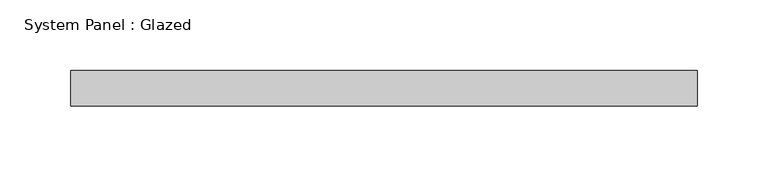
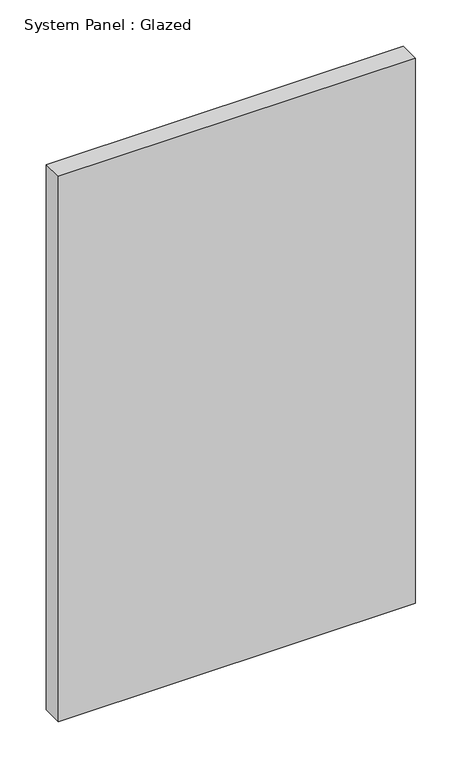
"""IFC4 building model written with IfcOpenShell, lengths in millimetres: plate geometry, System Panel : Glazed."""

from ifc_helpers import new_model, si_unit, origin, origin_with_axes, place, context, project, spatial, polyline, outline, extrude, source, transform, mapped, element, save


def system_panel_glazed_90648ddd(model_context):
    return source(origin(), model_context, "Body", "SweptSolid", [
        extrude(outline(polyline([(222.25, 19.05), (-222.25, 19.05), (-222.25, 44.45), (222.25, 44.45), (222.25, 19.05)])), origin_with_axes(), (0.0, 0.0, 1.0), 717.55),
    ])


if __name__ == "__main__":
    model = new_model("IFC4")
    model_context = context("Model", 3, world=origin())
    ifc_project = project(units=[si_unit("LENGTHUNIT", "METRE", prefix="MILLI")], contexts=[model_context])
    site = spatial("IfcSite", under=ifc_project)
    building = spatial("IfcBuilding", under=site)
    placement = place(None, origin())
    system_panel_glazed_shape = system_panel_glazed_90648ddd(model_context)
    element("IfcPlate", 1, ObjectType="System Panel : Glazed", at=placement, inside=building, context=model_context, shape_type="MappedRepresentation", body=[
        mapped(system_panel_glazed_shape, transform((0.0, 0.0, 0.0), x_axis=(1.0, 0.0, 0.0), y_axis=(0.0, 1.0, 0.0), z_axis=(0.0, 0.0, 1.0))),
    ])
    save(model, "model.ifc")

# Revit data of these elements
# Type "System Panel : Glazed"
#   Construction Type Id = "GSP4R"
#   Analytic Construction = "1/8 in Pilkington single glazing"
#   Visual Light Transmittance = 0.9
#   Solar Heat Gain Coefficient = 0.86
#   Heat Transfer Coefficient (U) = 1.18115 BTU/(h·ft²·°F)
#   Define Thermal Properties by = 1
# Element 1 (IfcPlate, "System Panel : Glazed")
#   Materials on its faces: "Glass"
# Materials
#   "Glass": class "Glass", colour RGB 0 128 192, transparency 0.75, Description = "Soda Lime Glass", Cost = 0
